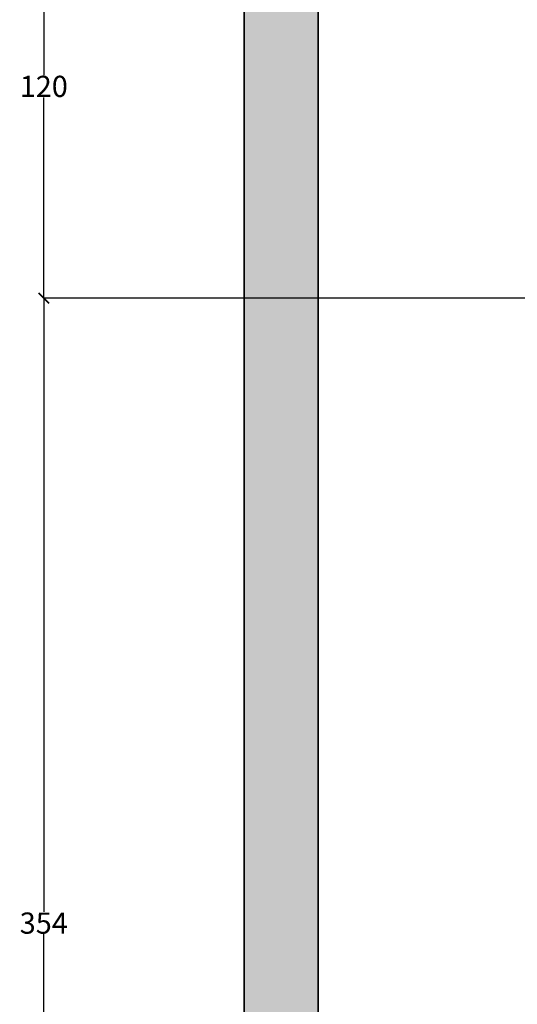
# Model space of a CAD drawing. Units: inches. Extents: x 925 to 2834, y 111 to 1355.
# Tile 13 of 25: x 928 to 1069, y 882 to 1160. Entities that reach past the tile are written whole.
import ezdxf

# ---------------------------------------------------------------- set-up
doc = ezdxf.new("R2010")
doc.units = ezdxf.units.IN
doc.header["$MEASUREMENT"] = 0
for name, color, linetype, lineweight in [('A-ANNO-DIMS', 2, 'Continuous', 18), ('A-ANNO-TTLB', 7, 'Continuous', 35), ('A-FLOR-PATT', 252, 'Continuous', 13)]:
    doc.layers.add(name, color=color, linetype=linetype, lineweight=lineweight)
doc.styles.get("Standard").update_dxf_attribs({"font": 'arial.ttf'})
doc.dimstyles.get("Standard").update_dxf_attribs({"dimtxt": 6, "dimasz": 3, "dimexe": 0.18, "dimexo": 0.0625, "dimgap": 0.09, "dimtad": 0, "dimtih": 1, "dimtoh": 1, "dimdec": 1, "dimzin": 0, "dimdsep": 46, "dimlunit": 3, "dimtxsty": 'Standard', "dimblk": 'ARCHTICK', "dimcen": 0.09, "dimadec": 0, "dimazin": 0, "dimtfac": 1, "dimtdec": 1, "dimtofl": 0, "dimtmove": 0, "dimatfit": 3, "dimfxl": 1, "dimtolj": 1, "dimtzin": 0, "dimarcsym": 0})

# ---------------------------------------------------------------- blocks, each defined once
blk = doc.blocks.new('_ArchTick')
at = {"color": 0, "linetype": 'ByBlock', "const_width": 0.15}
blk.add_lwpolyline([(-0.5, -0.5), (0.5, 0.5)], dxfattribs=at)
blk = doc.blocks.new('*D36')
at = {"layer": 'A-ANNO-DIMS', "color": 0, "lineweight": -2, "transparency": 16777216}
for p, q in [((1084.65, 1081.59), (934.81, 1081.59)), ((934.99, 1081.59), (934.99, 907.74)), ((934.99, 727.59), (934.99, 901.43)), ((1084.65, 727.59), (934.81, 727.59))]:
    blk.add_line(p, q, dxfattribs=at)
at = {"layer": 'Defpoints', "color": 0, "transparency": 16777216}
for p in [(934.99, 1081.59), (1084.71, 1081.59), (1084.71, 727.59)]:
    blk.add_point(p, dxfattribs=at)
at = {"layer": 'A-ANNO-DIMS', "color": 0, "lineweight": -2, "transparency": 16777216, "xscale": 3, "yscale": 3, "zscale": 3}
for p, rotation in [((934.99, 1081.59), 90), ((934.99, 727.59), 270)]:
    blk.add_blockref('_ArchTick', p, dxfattribs=dict(at, rotation=rotation))
at = {"layer": 'A-ANNO-DIMS', "color": 0, "transparency": 16777216, "insert": (934.99, 904.59), "char_height": 6, "attachment_point": 5}
blk.add_mtext('\\A1;354', dxfattribs=at)
blk = doc.blocks.new('*D37')
at = {"layer": 'A-ANNO-DIMS', "color": 0, "lineweight": -2, "transparency": 16777216}
for p, q in [((1084.65, 1201.59), (934.81, 1201.59)), ((934.99, 1201.59), (934.99, 1144.74)), ((934.99, 1081.59), (934.99, 1138.44)), ((1084.65, 1081.59), (934.81, 1081.59))]:
    blk.add_line(p, q, dxfattribs=at)
at = {"layer": 'Defpoints', "color": 0, "transparency": 16777216}
for p in [(934.99, 1201.59), (1084.71, 1201.59), (1084.71, 1081.59)]:
    blk.add_point(p, dxfattribs=at)
at = {"layer": 'A-ANNO-DIMS', "color": 0, "lineweight": -2, "transparency": 16777216, "xscale": 3, "yscale": 3, "zscale": 3}
for p, rotation in [((934.99, 1201.59), 90), ((934.99, 1081.59), 270)]:
    blk.add_blockref('_ArchTick', p, dxfattribs=dict(at, rotation=rotation))
at = {"layer": 'A-ANNO-DIMS', "color": 0, "transparency": 16777216, "insert": (934.99, 1141.59), "char_height": 6, "attachment_point": 5}
blk.add_mtext('\\A1;120', dxfattribs=at)

msp = doc.modelspace()

# ---------------------------------------------------------------- hatches: boundary and pattern name
at = {"layer": 'A-FLOR-PATT', "transparency": 33554605}
h = msp.add_hatch(color=256, dxfattribs=at)
h.dxf.hatch_style = 1
h.paths.add_polyline_path([(1931.688, 1294.5638), (991.7375, 1294.5638), (991.7375, 172.1134), (1931.688, 172.1134)])
h.paths.add_polyline_path([(1910.7128, 1273.5886), (1910.7128, 193.0886), (1012.7128, 193.0886), (1012.7128, 1273.5886)], flags=16)
h.paths.add_polyline_path([(1850.7128, 1213.5886), (1850.7128, 253.0886), (1072.7128, 253.0886), (1072.7128, 1213.5886)], flags=0)
h.paths.add_polyline_path([(1838.7128, 1201.5886), (1838.7128, 265.0886), (1084.7128, 265.0886), (1084.7128, 530.5886), (1084.7128, 1201.5886)], flags=0)
h.paths.add_polyline_path([(1547.6758, 1155.7396), (1547.6758, 1119.115), (1513.0687, 1119.115), (1513.0687, 1155.7396)], flags=0)
h.paths.add_polyline_path([(1600.1067, 1154.9439), (1634.7139, 1154.9439), (1634.7139, 1119.115), (1600.1067, 1119.115)], flags=0)
h.paths.add_polyline_path([(1505.2502, 1144.5358), (1505.2502, 1119.115), (1470.643, 1119.115), (1470.643, 1144.5358)], flags=0)
h.paths.add_polyline_path([(1559.1357, 1141.0962), (1593.7428, 1141.0962), (1593.7428, 1119.115), (1559.1357, 1119.115)], flags=0)
h.paths.add_polyline_path([(1462.8966, 1154.9439), (1462.8966, 1119.115), (1428.2895, 1119.115), (1428.2895, 1154.9439)], flags=0)
h.paths.add_polyline_path([(1642.4603, 1144.5358), (1677.0675, 1144.5358), (1677.0675, 1119.115), (1642.4603, 1119.115)], flags=0)
h.paths.add_polyline_path([(1422.3508, 1141.0962), (1422.3508, 1119.115), (1387.7436, 1119.115), (1387.7436, 1141.0962)], flags=0)
h.paths.add_polyline_path([(1684.8859, 1155.7396), (1719.4931, 1155.7396), (1719.4931, 1119.115), (1684.8859, 1119.115)], flags=0)
h.paths.add_polyline_path([(1718.7128, 1081.5886), (1718.7128, 1050.1249), (1715.7128, 1050.1249), (1715.7128, 1026.1249), (1715.7128, 1002.1249), (1718.7128, 1002.1249), (1730.7128, 1002.1249), (1730.7128, 998.1249), (1730.7128, 990.1249), (1730.7128, 986.1249), (1718.7128, 986.1249), (1718.7128, 893.5886), (1715.3735, 893.5886), (1715.3735, 891.5886), (1713.3735, 891.5886, 0.41421356), (1677.3735, 855.5886), (1713.3735, 855.5886), (1713.3735, 853.5886), (1715.3735, 853.5886), (1715.3735, 851.5886), (1718.7128, 851.5886), (1718.7128, 821.5865), (1734.4655, 821.5865), (1734.3735, 819.5886, -0.41421356), (1712.4415, 793.5886), (1712.4415, 791.5886), (1718.7128, 791.5886), (1718.7128, 717.5886), (1718.7128, 669.5886), (1732.7128, 669.5886), (1732.7128, 665.5886), (1732.7128, 641.5886), (1732.7128, 634.5886), (1732.7128, 610.5886), (1732.7128, 603.5886), (1718.7128, 603.5886), (1718.7128, 385.0886), (1434.2128, 385.0886), (1434.2128, 530.5886), (1410.2128, 530.5886), (1408.2128, 530.5886), (1408.2128, 532.5886, 0.41421356), (1372.2128, 568.5886), (1372.2128, 532.5886), (1370.2128, 532.5886), (1370.2128, 530.5886), (1368.2128, 530.5886), (1282.2128, 530.5886), (1210.2128, 530.5886), (1200.2128, 530.5886), (1200.2128, 542.1915), (1183.2307, 542.1915), (1183.2307, 546.1915), (1200.2128, 546.1915), (1200.2128, 572.1915), (1183.2307, 572.1915), (1183.2307, 576.1915), (1200.2128, 576.1915), (1200.2128, 727.5886), (1210.2128, 727.5886), (1234.2128, 727.5886), (1259.7128, 727.5886), (1259.7128, 775.5886), (1259.7128, 799.5886), (1259.7128, 847.5886), (1259.7128, 993.5872), (1259.7128, 1065.5872), (1259.7128, 1071.5886), (1219.6318, 1071.5886), (1219.6318, 1081.5886), (1084.7128, 1081.5886), (1084.7128, 1119.115), (1256.8974, 1119.115), (1256.8974, 1154.9439), (1291.5046, 1154.9439), (1291.5046, 1119.115), (1256.8974, 1119.115), (1256.6723, 1081.5886), (1293.7128, 1081.5886), (1341.7128, 1081.5886), (1341.7128, 1093.5886), (1347.7128, 1093.5886), (1371.7128, 1093.5886), (1377.7128, 1093.5886), (1377.7128, 1081.5886), (1668.7128, 1081.5886), (1668.7128, 1117.5886), (1675.7128, 1117.5886), (1711.7128, 1117.5886), (1718.7128, 1117.5886)], flags=0)
h.paths.add_polyline_path([(1376.2838, 1155.7396), (1376.2838, 1119.115), (1341.6766, 1119.115), (1341.6766, 1155.7396)], flags=0)
h.paths.add_polyline_path([(1341.7128, 1076.0886), (1293.7128, 1076.0886), (1293.7128, 1071.5886), (1269.7128, 1071.5886), (1269.7128, 1065.5872), (1266.7128, 1065.5872), (1266.7128, 1029.5872), (1265.7128, 1029.5872), (1265.7128, 993.5872), (1269.7128, 993.5872), (1269.7128, 903.5886), (1269.7128, 893.5886), (1269.7128, 847.5886), (1265.2128, 847.5886), (1265.2128, 799.5886), (1269.7128, 799.5886), (1269.7128, 775.5886), (1265.2128, 775.5886), (1265.2128, 727.5886), (1269.7128, 727.5886), (1444.2128, 727.5886), (1444.2128, 717.5886), (1234.2128, 717.5886), (1234.2128, 722.0886), (1210.2128, 722.0886), (1210.2128, 717.5886), (1210.2128, 540.5886), (1210.2128, 536.0886), (1282.2128, 536.0886), (1282.2128, 535.0886), (1210.2128, 535.0886), (1210.2128, 540.5886), (1210.2128, 717.5886), (1210.2128, 723.0886), (1234.2128, 723.0886), (1234.2128, 717.5886), (1444.2128, 717.5886), (1444.2128, 727.5886), (1269.7128, 727.5886), (1264.2128, 727.5886), (1264.2128, 775.5886), (1269.7128, 775.5886), (1269.7128, 799.5886), (1264.2128, 799.5886), (1264.2128, 847.5886), (1269.7128, 847.5886), (1269.7128, 893.5886), (1269.7128, 903.5886), (1269.7128, 993.5872), (1264.7128, 993.5872), (1264.7128, 1029.5872), (1265.7128, 1029.5872), (1265.7128, 1065.5872), (1269.7128, 1065.5872), (1269.7128, 1071.5886), (1293.7128, 1071.5886), (1293.7128, 1077.0886), (1341.7128, 1077.0886)], flags=0)
h.paths.add_polyline_path([(1730.9529, 1141.0962), (1765.5601, 1141.0962), (1765.5601, 1119.115), (1730.9529, 1119.115)], flags=0)
h.paths.add_polyline_path([(1333.8582, 1144.5358), (1333.8582, 1119.115), (1299.251, 1119.115), (1299.251, 1144.5358)], flags=0)
h.paths.add_polyline_path([(1592.7128, 968.5886), (1596.0342, 968.5886), (1602.7128, 968.5886), (1708.7128, 968.5886), (1708.7128, 903.5886), (1602.7128, 903.5886), (1602.7128, 938.5886), (1592.7128, 938.5886), (1592.7128, 903.5886), (1451.7128, 903.5886), (1451.7128, 893.5886), (1511.7128, 893.5886), (1511.7128, 881.5886), (1515.2128, 881.5886), (1518.7128, 881.5886), (1518.7128, 893.5886), (1592.7128, 893.5886), (1592.7128, 799.5886), (1518.7128, 799.5886), (1518.7128, 857.5886), (1511.7128, 857.5886), (1511.7128, 799.5886), (1511.7128, 772.0886), (1521.7128, 772.0886), (1521.7128, 792.5886), (1592.7128, 792.5886), (1592.7128, 727.5886), (1521.7128, 727.5886), (1521.7128, 748.0886), (1511.7128, 748.0886), (1511.7128, 717.5886), (1708.7128, 717.5886), (1714.2128, 717.5886), (1714.2128, 669.5886), (1708.7128, 669.5886), (1708.7128, 641.5886), (1492.2128, 641.5886), (1492.2128, 631.5886), (1621.2128, 631.5886), (1621.2128, 443.0886), (1625.7128, 443.0886), (1625.7128, 503.0886), (1625.7128, 507.5886), (1625.7128, 631.5886), (1708.7128, 631.5886), (1708.7128, 507.5886), (1655.7128, 507.5886), (1655.7128, 503.0886), (1708.7128, 503.0886), (1708.7128, 395.0886), (1625.7128, 395.0886), (1625.7128, 419.0886), (1621.2128, 419.0886), (1621.2128, 395.0886), (1482.2128, 395.0886), (1482.2128, 385.0886), (1434.2128, 385.0886), (1434.2128, 433.0886), (1444.2128, 433.0886), (1444.2128, 631.5886), (1450.2128, 631.5886), (1450.2128, 634.91), (1452.2128, 634.91), (1452.2128, 669.5886), (1454.2128, 669.5886, -0.40021217), (1490.1712, 635.3173), (1492.2128, 635.3173), (1492.2128, 641.5886), (1564.7128, 641.5886), (1564.7128, 677.5886), (1672.7128, 677.5886), (1672.7128, 681.5886), (1564.7128, 681.5886), (1564.7128, 717.5886), (1511.7128, 717.5886), (1511.7128, 748.0886), (1511.7128, 772.0886), (1511.7128, 799.5886), (1511.7128, 857.5886), (1511.8913, 857.5886), (1511.8913, 859.5886), (1515.6201, 859.5886, 0.41421356), (1537.552, 879.5886), (1513.552, 879.5886), (1511.8913, 879.5886), (1511.8913, 881.5886), (1511.7128, 881.5886), (1511.7128, 893.5886), (1451.7128, 893.5886), (1451.7128, 903.5886), (1592.7128, 903.5886), (1592.7128, 938.5886), (1592.7128, 940.5886), (1596.4415, 940.5886, 0.41421356), (1618.3735, 966.5886), (1594.3735, 966.5886), (1592.7128, 966.5886)], flags=0)
h.paths.add_polyline_path([(1377.7128, 903.5886), (1377.7128, 893.5886), (1305.7128, 893.5886), (1305.7128, 903.5886)], flags=0)
h.paths.add_polyline_path([(1708.7128, 821.5886), (1712.0342, 821.5886), (1712.0342, 819.5886), (1710.3735, 819.5886), (1708.7128, 819.5886)], flags=0)
h.paths.add_polyline_path([(1576.7128, 695.1992), (1575.5896, 693.6649), (1575.9687, 694.6994), (1575.4438, 695.1992), (1575.9687, 695.699), (1575.5896, 696.7335)], flags=0)
h.paths.add_polyline_path([(1565.9817, 662.3134), (1565.4568, 661.8136), (1565.8359, 660.7791), (1564.7128, 662.3134), (1565.8359, 663.8477), (1565.4568, 662.8132)], flags=0)
h.paths.add_polyline_path([(1444.2128, 433.0886), (1444.2128, 395.0886), (1482.2128, 395.0886), (1482.2128, 389.0886), (1438.2128, 389.0886), (1438.2128, 391.8608), (1438.2128, 433.0886)], flags=0)
h.paths.add_polyline_path([(1410.2128, 506.5886), (1410.2128, 289.0886), (1108.7128, 289.0886), (1108.7128, 506.5886)], flags=0)
h.paths.add_polyline_path([(1612.3153, 838.3016), (1680.4151, 838.3016), (1680.4151, 851.3131), (1612.3153, 851.3131)], flags=8)
h.paths.add_polyline_path([(1208.3174, 395.0436), (1282.1017, 395.0436), (1282.1017, 408.0552), (1208.3174, 408.0552)], flags=8)
h.paths.add_polyline_path([(1291.8049, 598.7427), (1369.8017, 598.7427), (1369.8017, 611.7542), (1291.8049, 611.7542)], flags=8)
h.paths.add_polyline_path([(1119.679, 917.3022), (1191.0817, 917.3022), (1191.0817, 930.3137), (1119.679, 930.3137)], flags=8)
h.paths.add_polyline_path([(1332.2261, 815.9808), (1410.2258, 815.9808), (1410.2258, 829.001), (1332.2261, 829.001)], flags=8)
h.paths.add_polyline_path([(1390.9013, 955.8158), (1475.4981, 955.8158), (1475.4981, 968.8273), (1390.9013, 968.8273)], flags=8)
h.paths.add_polyline_path([(1620.3436, 998.9325), (1688.4434, 998.9325), (1688.4434, 1011.944), (1620.3436, 1011.944)], flags=8)
h.paths.add_polyline_path([(1620.3436, 914.1039), (1691.7405, 914.1039), (1691.7405, 927.1155), (1620.3436, 927.1155)], flags=8)
h.paths.add_polyline_path([(1521.4542, 816.005), (1589.5569, 816.005), (1589.5569, 829.0253), (1521.4542, 829.0253)], flags=8)
h.paths.add_polyline_path([(1528.524, 740.3497), (1602.3082, 740.3497), (1602.3082, 753.3613), (1528.524, 753.3613)], flags=8)
h.paths.add_polyline_path([(1627.6094, 762.6128), (1702.3091, 762.6128), (1702.3091, 775.6244), (1627.6094, 775.6244)], flags=8)
h.paths.add_polyline_path([(1610.5442, 657.2751), (1684.3284, 657.2751), (1684.3284, 670.2867), (1610.5442, 670.2867)], flags=8)
h.paths.add_polyline_path([(1636.6983, 519.472), (1711.3981, 519.472), (1711.3981, 532.4835), (1636.6983, 532.4835)], flags=8)
h.paths.add_polyline_path([(1616.8577, 424.8539), (1694.8545, 424.8539), (1694.8545, 437.8654), (1616.8577, 437.8654)], flags=8)
h.paths.add_polyline_path([(1506.1456, 460.8838), (1579.9299, 460.8838), (1579.9299, 473.8953), (1506.1456, 473.8953)], flags=8)
h.paths.add_polyline_path([(1624.6119, 784.6011), (1696.9185, 784.6011), (1696.9185, 797.7864), (1624.6119, 797.7864)], flags=8)
h.paths.add_polyline_path([(1606.3732, 854.2194), (1683.3039, 854.2194), (1683.3039, 867.4048), (1606.3732, 867.4048)], flags=8)
h.paths.add_polyline_path([(1127.8008, 940.3581), (1165.1637, 940.3581), (1165.1637, 953.5348), (1127.8008, 953.5348)], flags=8)
h.paths.add_polyline_path([(1620.8657, 1019.4968), (1677.3447, 1019.4968), (1677.3447, 1032.6735), (1620.8657, 1032.6735)], flags=8)
h.paths.add_polyline_path([(1620.8643, 930.1821), (1703.0564, 930.1821), (1703.0564, 943.3675), (1620.8643, 943.3675)], flags=8)
h.paths.add_polyline_path([(1324.5702, 836.8338), (1408.0892, 836.8338), (1408.0892, 850.0191), (1324.5702, 850.0191)], flags=8)
h.paths.add_polyline_path([(1281.6584, 622.8885), (1383.6213, 622.8885), (1383.6213, 636.0739), (1281.6584, 636.0739)], flags=8)
h.paths.add_polyline_path([(1210.6721, 416.7893), (1269.1299, 416.7893), (1269.1299, 429.9747), (1210.6721, 429.9747)], flags=8)
h.paths.add_polyline_path([(1507.8264, 477.4836), (1586.7329, 477.4836), (1586.7329, 490.669), (1507.8264, 490.669)], flags=8)
h.paths.add_polyline_path([(1643.6238, 443.8135), (1696.6696, 443.8135), (1696.6696, 456.5643), (1643.6238, 456.5643)], flags=8)
h.paths.add_polyline_path([(1647.2466, 540.5638), (1693.1825, 540.5638), (1693.1825, 553.7491), (1647.2466, 553.7491)], flags=8)
h.paths.add_polyline_path([(1626.0633, 668.5064), (1673.3174, 668.5064), (1673.3174, 681.6831), (1626.0633, 681.6831)], flags=8)
h.paths.add_polyline_path([(1538.2915, 830.7872), (1567.5942, 830.7872), (1567.5942, 843.5293), (1538.2915, 843.5293)], flags=8)
h.paths.add_polyline_path([(1530.9338, 754.0477), (1559.576, 754.0477), (1559.576, 766.7898), (1530.9338, 766.7898)], flags=8)
h.paths.add_polyline_path([(1351.2461, 979.2309), (1513.8919, 979.2309), (1513.8919, 992.4076), (1351.2461, 992.4076)], flags=8)

# ---------------------------------------------------------------- linework, layer by layer
at = {"layer": 'A-ANNO-TTLB'}
for points in [[(991.7375, 172.1134), (1931.688, 172.1134), (1931.688, 1294.5638), (991.7375, 1294.5638)], [(1012.7128, 193.0886), (1910.7128, 193.0886), (1910.7128, 1273.5886), (1012.7128, 1273.5886)]]:
    msp.add_lwpolyline(points, close=True, dxfattribs=at)

# ---------------------------------------------------------------- dimensions: what is measured, and where the dimension line sits
at = {"layer": 'A-ANNO-DIMS'}
for base, p1, p2, picture, middle in [((934.9875, 1201.5886), (1084.7128, 1081.5886), (1084.7128, 1201.5886), '*D37', (934.9875, 1141.5886)), ((934.9875, 1081.5886), (1084.7128, 727.5886), (1084.7128, 1081.5886), '*D36', (934.9875, 904.5886))]:
    dim = msp.add_linear_dim(base=base, p1=p1, p2=p2, angle=90, dimstyle='Standard', override={"dimdec": 0, "dimlfac": 1, "dimrnd": 0, "dimzin": 0, "dimdsep": 46, "dimlunit": 2}, dxfattribs=at)
    dim.commit()
    dim.dimension.update_dxf_attribs({"geometry": picture, "text_midpoint": middle})

doc.saveas('drawing.dxf')
